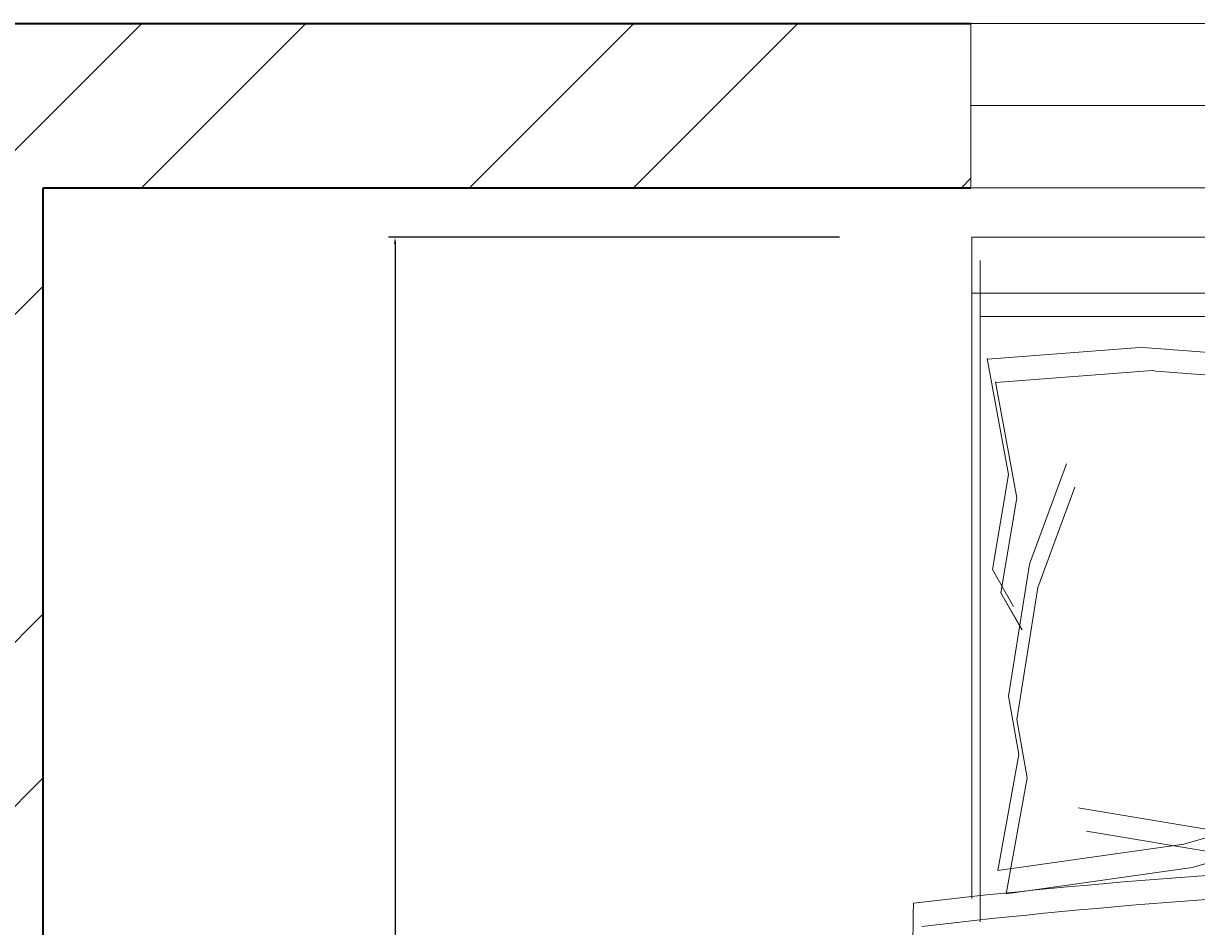
# Model space of a CAD drawing. Units: inches. Extents: x 1885 to 2748, y 783 to 2421.
# Tile 97 of 117: x 2363 to 2395, y 2328 to 2353. Entities that reach past the tile are written whole.
import ezdxf

# ---------------------------------------------------------------- set-up
doc = ezdxf.new("R2010")
doc.units = ezdxf.units.IN
for name, color, linetype, lineweight in [('A-ANNO-DIMS', 2, 'Continuous', 18), ('A-FURN', 8, 'Continuous', 13), ('A-GLAZ', 181, 'Continuous', 18), ('A-WALL', 7, 'Continuous', 35)]:
    doc.layers.add(name, color=color, linetype=linetype, lineweight=lineweight)
doc.layers.add('A-WALL-PATT', color=85, linetype='Continuous', lineweight=13, true_color=0x58ba48)
doc.styles.get("Standard").update_dxf_attribs({"font": 'arial.ttf'})
doc.dimstyles.get("Standard").update_dxf_attribs({"dimtxt": 0.18, "dimasz": 0.18, "dimexe": 0.18, "dimexo": 0.0625, "dimgap": 0.09, "dimtad": 0, "dimtih": 1, "dimtoh": 1, "dimdec": 4, "dimzin": 0, "dimdsep": 46, "dimtxsty": 'Standard', "dimcen": 0.09, "dimadec": 0, "dimazin": 0, "dimtfac": 1, "dimtdec": 4, "dimtofl": 0, "dimtmove": 0, "dimatfit": 3, "dimfxl": 1, "dimtolj": 1, "dimtzin": 0, "dimarcsym": 0})

# ---------------------------------------------------------------- blocks, each defined once
blk = doc.blocks.new('BED-DOUBLE')
for p, q in [((0.004, 3.474), (0.004, 51.493)), ((2.177, 3.702), (2.177, 51.493)), ((2.177, 3.702), (2.177, 51.492)), ((1.537, 3.474), (1.537, 51.264)), ((1.537, 3.474), (1.537, 51.264)), ((3.67, 8.512), (3.959, 12.335)), ((3.67, 8.512), (3.959, 12.335)), ((3.031, 8.284), (3.32, 12.107)), ((3.031, 8.283), (3.32, 12.107)), ((16.271, 6.609), (16.938, 10.641)), ((16.272, 6.609), (16.938, 10.64)), ((16.938, 10.641), (17.261, 9.508)), ((16.938, 10.64), (17.261, 9.507)), ((15.632, 6.38), (16.299, 10.412)), ((15.632, 6.38), (16.299, 10.412)), ((16.299, 10.412), (16.622, 9.279)), ((16.299, 10.412), (16.622, 9.279)), ((17.261, 9.508), (17.984, 4.411)), ((17.261, 9.507), (17.984, 4.411)), ((16.622, 9.279), (17.345, 4.183)), ((16.622, 9.279), (17.345, 4.182)), ((3.652, 8.407), (3.67, 8.512)), ((3.652, 8.406), (3.67, 8.512)), ((3.981, 4.126), (3.652, 8.407)), ((3.981, 4.125), (3.652, 8.406)), ((3.012, 8.178), (3.031, 8.284)), ((3.012, 8.178), (3.031, 8.283)), ((3.342, 3.897), (3.012, 8.178)), ((3.342, 3.897), (3.012, 8.178)), ((9.598, 5.278), (6.851, 6.29)), ((9.598, 5.278), (6.851, 6.29)), ((8.959, 5.05), (6.211, 6.062)), ((8.959, 5.05), (6.211, 6.061)), ((13.213, 4.7), (9.598, 5.278)), ((13.213, 4.7), (9.598, 5.278)), ((12.573, 4.472), (8.959, 5.05)), ((12.573, 4.471), (8.959, 5.05)), ((9.743, 4.266), (10.755, 4.845)), ((9.743, 4.266), (10.755, 4.844)), ((14.803, 4.989), (13.213, 4.7)), ((14.803, 4.989), (13.213, 4.7)), ((17.984, 4.411), (14.803, 4.989)), ((17.984, 4.411), (14.803, 4.989)), ((3.959, 4.122), (7.14, 4.7)), ((3.959, 4.121), (7.14, 4.7)), ((7.14, 4.7), (9.743, 4.266)), ((7.14, 4.7), (9.743, 4.266)), ((9.103, 4.038), (10.115, 4.616)), ((9.103, 4.038), (10.115, 4.616)), ((14.164, 4.761), (12.573, 4.472)), ((14.164, 4.76), (12.573, 4.471)), ((17.345, 4.183), (14.164, 4.761)), ((17.345, 4.182), (14.164, 4.76)), ((3.32, 3.893), (6.501, 4.472)), ((3.32, 3.893), (6.501, 4.471)), ((6.501, 4.472), (9.103, 4.038)), ((6.501, 4.471), (9.103, 4.038)), ((18.753, 3.702), (0.643, 3.702)), ((18.753, 3.702), (0.643, 3.702)), ((18.114, 3.474), (0.004, 3.474)), ((18.114, 3.474), (0.004, 3.474))]:
    blk.add_line(p, q)
for centre, radius, start, end in [((182.695, 21.586), 164.969, 176.08655, 186.78213), ((182.695, 21.586), 164.969, 176.08655, 186.78213), ((182.056, 21.358), 164.969, 176.08655, 186.78213), ((182.056, 21.357), 164.969, 176.08655, 186.78213), ((20.1, 85.16), 83.306, 268.72178, 275.60397), ((20.1, 85.16), 83.306, 268.72178, 275.60397)]:
    blk.add_arc(centre, radius, start, end)
blk = doc.blocks.new('WIN-60')
for p, q in [((0.004, 59.998), (0.004, -0.002)), ((2.254, 59.998), (2.254, -0.002)), ((4.504, -0.002), (4.504, 59.998)), ((2.254, -0.002), (0.004, -0.002)), ((0.004, -0.002), (4.504, -0.002))]:
    blk.add_line(p, q)
blk = doc.blocks.new('*D27')
at = {"layer": 'A-ANNO-DIMS', "color": 0, "lineweight": -2, "transparency": 16777216}
for p, q in [((2385.079, 2346.649), (2372.729, 2346.649)), ((2372.909, 2346.469), (2372.909, 2306.056)), ((2372.909, 2265.28), (2372.909, 2305.693)), ((2385.079, 2265.1), (2372.729, 2265.1))]:
    blk.add_line(p, q, dxfattribs=at)
at = {"layer": 'A-ANNO-DIMS', "color": 0, "transparency": 16777216}
for points in [[(2372.879, 2346.469), (2372.939, 2346.469), (2372.909, 2346.649)], [(2372.879, 2265.28), (2372.939, 2265.28), (2372.909, 2265.1)]]:
    blk.add_solid(points, dxfattribs=at)
at = {"layer": 'Defpoints', "color": 0, "transparency": 16777216}
for p in [(2385.141, 2346.649), (2372.909, 2265.1), (2385.141, 2265.1)]:
    blk.add_point(p, dxfattribs=at)
at = {"layer": 'A-ANNO-DIMS', "color": 0, "transparency": 16777216, "insert": (2372.909, 2305.874), "char_height": 0.18, "attachment_point": 5}
blk.add_mtext('\\A1;BED 82 TYP.', dxfattribs=at)

msp = doc.modelspace()

# ---------------------------------------------------------------- hatches: boundary and pattern name
at = {"layer": 'A-WALL-PATT'}
h = msp.add_hatch(dxfattribs=at)
h.set_pattern_fill('ANSI32', color=256)
h.paths.add_polyline_path([(2007.772, 2318.006), (1980.774, 2318.006), (1980.774, 2281.215), (1985.274, 2281.215), (1985.274, 2313.506), (2007.772, 2313.506), (2007.772, 2315.756)])
h.paths.add_polyline_path([(2094.324, 2318.006), (2067.772, 2318.006), (2067.772, 2313.506), (2094.324, 2313.506), (2094.324, 2315.756)])
h.paths.add_polyline_path([(2131.367, 2315.756), (2131.367, 2318.006), (2131.189, 2318.006), (2112.609, 2318.006), (2112.609, 2313.506), (2117.274, 2313.506), (2117.274, 2255.201), (2121.774, 2255.201), (2121.774, 2313.506), (2131.367, 2313.506)])
h.paths.add_polyline_path([(2190.512, 2318.006), (2155.367, 2318.006), (2155.367, 2313.506), (2169.774, 2313.506), (2169.774, 2229.506), (2121.774, 2229.506), (2121.774, 2233.451), (2119.524, 2233.451), (2117.274, 2233.451), (2117.274, 2201.101), (2121.774, 2201.101), (2121.774, 2225.006), (2169.774, 2225.006), (2169.774, 2165.006), (2306.274, 2165.006), (2306.274, 2066.006), (2310.774, 2066.006), (2344.274, 2066.006), (2486.274, 2066.006), (2486.274, 1886.006), (2483.02, 1886.006), (2483.02, 1881.506), (2486.274, 1881.506), (2486.274, 1880.678), (2490.774, 1880.678), (2490.774, 2070.506), (2344.274, 2070.506), (2310.774, 2070.506), (2310.774, 2165.006), (2310.774, 2173.636), (2308.524, 2173.636), (2306.274, 2173.636), (2306.274, 2169.506), (2174.274, 2169.506), (2174.274, 2313.506), (2190.512, 2313.506), (2190.512, 2315.756)])
h.paths.add_polyline_path([(1985.274, 2221.215), (1980.774, 2221.215), (1980.774, 2165.006), (1992.774, 2165.006), (1992.774, 2141.927), (1997.274, 2141.927), (1997.274, 2165.006), (2117.274, 2165.006), (2117.274, 2163.126), (2121.774, 2163.126), (2121.774, 2172.734), (2119.524, 2172.734), (2117.274, 2172.734), (2117.274, 2169.506), (1985.274, 2169.506)])
h.paths.add_polyline_path([(1997.274, 2105.927), (1992.774, 2105.927), (1992.774, 2070.506), (2016.774, 2070.506), (2016.774, 2059.123), (2019.024, 2059.123), (2021.274, 2059.123), (2021.274, 2070.506), (2117.274, 2070.506), (2117.274, 2022.506), (2114.423, 2022.506), (2114.423, 2018.006), (2123.627, 2018.006), (2123.627, 2020.256), (2123.627, 2022.506), (2121.774, 2022.506), (2121.774, 2142.587), (2119.524, 2142.587), (2117.274, 2142.587), (2117.274, 2075.006), (1997.274, 2075.006)])
h.paths.add_polyline_path([(2092.029, 2020.256), (2092.029, 2022.506), (2021.274, 2022.506), (2021.274, 2035.123), (2016.774, 2035.123), (2016.774, 2018.006), (2016.774, 1978.784), (2021.274, 1978.784), (2021.274, 2018.006), (2092.029, 2018.006)])
h.paths.add_polyline_path([(2260.938, 2022.506), (2153.105, 2022.506), (2153.105, 2020.256), (2153.105, 2018.006), (2155.274, 2018.006), (2155.274, 1886.006), (2107.629, 1886.006), (2107.629, 1881.506), (2182.911, 1881.506), (2182.911, 1883.756), (2182.911, 1886.006), (2159.774, 1886.006), (2159.774, 2018.006), (2260.938, 2018.006), (2260.938, 2020.256)])
h.paths.add_polyline_path([(2047.629, 1883.756), (2047.629, 1886.006), (2021.274, 1886.006), (2021.274, 1918.784), (2019.024, 1918.784), (2016.774, 1918.784), (2016.774, 1881.506), (2047.629, 1881.506)])
h.paths.add_polyline_path([(2306.361, 1883.756), (2306.361, 1886.006), (2296.274, 1886.006), (2296.274, 1982.006), (2316.535, 1982.006), (2316.535, 1984.256), (2316.535, 1986.506), (2296.274, 1986.506), (2296.274, 2022.506), (2289.276, 2022.506), (2289.276, 2018.006), (2291.774, 2018.006), (2291.774, 1886.006), (2242.911, 1886.006), (2242.911, 1881.506), (2306.361, 1881.506)], flags=17)
h.paths.add_polyline_path([(1985.274, 1843.006), (2021.6, 1843.006), (2021.534, 1845.441), (2021.477, 1847.506), (1980.774, 1847.506), (1980.774, 1809.446), (1985.274, 1809.446)])
h.paths.add_polyline_path([(2131.482, 1845.256), (2131.482, 1847.506), (2081.534, 1847.506), (2081.534, 1843.006), (2117.274, 1843.006), (2117.274, 1784.147), (2119.524, 1784.147), (2121.774, 1784.147), (2121.774, 1843.006), (2131.482, 1843.006)])
h.paths.add_polyline_path([(2203.886, 1847.506), (2155.482, 1847.506), (2155.482, 1843.006), (2169.774, 1843.006), (2169.774, 1759.006), (2121.774, 1759.006), (2121.774, 1761.457), (2117.274, 1761.457), (2117.274, 1730.429), (2121.774, 1730.429), (2121.774, 1754.506), (2177.421, 1754.506), (2177.421, 1756.756), (2177.421, 1759.006), (2174.274, 1759.006), (2174.274, 1843.006), (2203.886, 1843.006)])
h.paths.add_polyline_path([(2335.554, 1845.256), (2335.554, 1847.506), (2239.886, 1847.506), (2239.886, 1843.006), (2306.274, 1843.006), (2306.274, 1759.006), (2199.486, 1759.006), (2199.486, 1754.506), (2310.774, 1754.506), (2310.774, 1843.006), (2335.554, 1843.006)])
h.paths.add_polyline_path([(2348.774, 2022.506), (2344.274, 2022.506), (2344.274, 1986.506), (2341.681, 1986.506), (2341.681, 1982.006), (2344.274, 1982.006), (2344.274, 1886.006), (2330.361, 1886.006), (2330.361, 1881.506), (2361.627, 1881.506), (2361.627, 1883.756), (2361.627, 1886.006), (2348.774, 1886.006)], flags=17)
h.paths.add_polyline_path([(2283.251, 2315.756), (2283.251, 2318.006), (2238.512, 2318.006), (2238.512, 2313.506), (2283.251, 2313.506)], flags=17)
h.paths.add_polyline_path([(2363.274, 2348.006), (2388.677, 2348.006), (2388.677, 2350.256), (2388.677, 2352.506), (2358.774, 2352.506), (2358.774, 2348.006), (2358.774, 2318.006), (2344.481, 2318.006), (2344.481, 2313.506), (2358.774, 2313.506), (2358.774, 2229.506), (2310.774, 2229.506), (2310.774, 2231.952), (2306.274, 2231.952), (2306.274, 2205.611), (2310.774, 2205.611), (2310.774, 2225.006), (2358.774, 2225.006), (2358.774, 2211.506), (2452.329, 2211.506), (2452.329, 2213.756), (2452.329, 2216.006), (2363.274, 2216.006), (2363.274, 2318.006)])
h.paths.add_polyline_path([(2310.774, 2313.506), (2320.481, 2313.506), (2320.481, 2315.756), (2320.481, 2318.006), (2302.728, 2318.006), (2302.728, 2313.506), (2306.274, 2313.506), (2306.274, 2251.076), (2310.774, 2251.076)], flags=17)
h.paths.add_polyline_path([(2490.774, 2352.506), (2486.274, 2352.506), (2448.677, 2352.506), (2448.677, 2348.006), (2486.274, 2348.006), (2486.274, 2318.006), (2486.274, 2216.006), (2481.78, 2216.006), (2481.78, 2211.506), (2486.274, 2211.506), (2486.274, 2165.006), (2493.289, 2165.006), (2493.289, 2167.256), (2493.289, 2169.506), (2490.774, 2169.506), (2490.774, 2313.506), (2494.429, 2313.506), (2494.429, 2318.006), (2490.774, 2318.006)])
h.paths.add_polyline_path([(2534.653, 2318.006), (2515.691, 2318.006), (2515.691, 2313.506), (2534.653, 2313.506), (2534.653, 2315.756)])
h.paths.add_polyline_path([(2618.274, 2318.006), (2594.653, 2318.006), (2594.653, 2313.506), (2613.774, 2313.506), (2613.774, 2281.706), (2618.274, 2281.706)])
h.paths.add_polyline_path([(2618.274, 2221.706), (2613.774, 2221.706), (2613.774, 2169.506), (2554.019, 2169.506), (2554.019, 2165.006), (2613.774, 2165.006), (2613.774, 2152.878), (2618.274, 2152.878)])
h.paths.add_polyline_path([(2618.274, 2128.878), (2616.024, 2128.878), (2613.774, 2128.878), (2613.774, 2117.006), (2529.774, 2117.006), (2529.774, 2165.006), (2532.848, 2165.006), (2532.848, 2169.506), (2522.867, 2169.506), (2522.867, 2165.006), (2525.274, 2165.006), (2525.274, 2117.006), (2525.274, 2112.506), (2525.274, 2108.576), (2529.774, 2108.576), (2529.774, 2112.506), (2613.774, 2112.506), (2613.774, 2080.19), (2618.274, 2080.19)])
h.paths.add_polyline_path([(2618.274, 2044.19), (2616.024, 2044.19), (2613.774, 2044.19), (2613.774, 2015.506), (2529.774, 2015.506), (2529.774, 2088.582), (2527.524, 2088.582), (2525.274, 2088.582), (2525.274, 2011.006), (2613.774, 2011.006), (2613.774, 1956.755), (2618.274, 1956.755)])
h.paths.add_polyline_path([(2618.274, 1881.506), (2618.274, 1896.755), (2613.774, 1896.755), (2613.774, 1881.506), (2613.774, 1847.506), (2592.715, 1847.506), (2592.715, 1843.006), (2613.774, 1843.006), (2613.774, 1765.006), (2613.774, 1760.506), (2609.621, 1760.506), (2609.621, 1756.006), (2613.774, 1756.006), (2613.774, 1660.006), (2608.544, 1660.006), (2608.544, 1655.506), (2613.774, 1655.506), (2613.774, 1508.158), (2618.274, 1508.158)])
h.paths.add_polyline_path([(2565.774, 1843.006), (2568.997, 1843.006), (2568.997, 1847.506), (2490.774, 1847.506), (2490.774, 1849.7), (2488.524, 1849.7), (2486.274, 1849.7), (2486.274, 1847.506), (2477.274, 1847.506), (2477.274, 1838.506), (2477.274, 1821.493), (2486.274, 1821.493), (2486.274, 1838.506), (2561.274, 1838.506), (2561.274, 1765.006), (2486.274, 1765.006), (2486.274, 1786.157), (2477.274, 1786.157), (2477.274, 1765.006), (2477.274, 1756.006), (2486.274, 1756.006), (2565.774, 1756.006), (2585.621, 1756.006), (2585.621, 1758.256), (2585.621, 1760.506), (2565.774, 1760.506), (2565.774, 1765.006)])
h.paths.add_polyline_path([(2486.274, 1651.006), (2561.274, 1651.006), (2561.274, 1567.006), (2486.274, 1567.006), (2486.274, 1591.321), (2477.274, 1591.321), (2477.274, 1567.006), (2477.274, 1558.006), (2477.274, 1555.439), (2481.774, 1555.439), (2481.774, 1558.006), (2568.653, 1558.006), (2568.653, 1560.256), (2568.653, 1562.506), (2565.774, 1562.506), (2565.774, 1655.506), (2584.544, 1655.506), (2584.544, 1657.756), (2584.544, 1660.006), (2565.774, 1660.006), (2486.274, 1660.006), (2477.274, 1660.006), (2477.274, 1651.006), (2477.274, 1632.989), (2486.274, 1632.989)])
h.paths.add_polyline_path([(2449.967, 1883.756), (2449.967, 1886.006), (2421.627, 1886.006), (2421.627, 1881.506), (2449.967, 1881.506)], flags=17)
h.paths.add_polyline_path([(2447.274, 1847.506), (2395.554, 1847.506), (2395.554, 1843.006), (2442.774, 1843.006), (2442.774, 1809.27), (2447.274, 1809.27)])
h.paths.add_polyline_path([(1985.274, 1749.446), (1980.774, 1749.446), (1980.774, 1694.504), (1985.274, 1694.504), (1985.274, 1694.506), (1986.897, 1694.506), (1986.897, 1697.78), (1986.897, 1699.006), (1985.274, 1699.006)])
h.paths.add_polyline_path([(2152.774, 1699.006), (2121.774, 1699.006), (2121.774, 1703.668), (2119.524, 1703.668), (2117.274, 1703.668), (2117.274, 1699.006), (2009.219, 1699.006), (2009.219, 1694.506), (2148.274, 1694.506), (2148.274, 1692.631), (2152.774, 1692.631)])
h.paths.add_polyline_path([(2016.274, 1694.506), (2011.774, 1694.506), (2011.774, 1558.006), (2040.806, 1558.006), (2040.806, 1560.256), (2040.806, 1562.506), (2016.274, 1562.506)])
h.paths.add_polyline_path([(2152.774, 1663.017), (2150.524, 1663.017), (2148.274, 1663.017), (2148.274, 1562.506), (2100.806, 1562.506), (2100.806, 1558.006), (2165.119, 1558.006), (2165.119, 1560.256), (2165.119, 1562.506), (2152.774, 1562.506), (2152.774, 1610.506), (2224.774, 1610.506), (2224.774, 1607.99), (2229.274, 1607.99), (2229.274, 1615.006), (2152.774, 1615.006)])
h.paths.add_polyline_path([(2238.613, 1560.256), (2238.613, 1562.506), (2229.274, 1562.506), (2229.274, 1588.756), (2227.024, 1588.763), (2224.774, 1588.771), (2224.774, 1562.506), (2189.119, 1562.506), (2189.119, 1558.006), (2238.613, 1558.006)])
h.paths.add_polyline_path([(2336.024, 1560.256), (2336.024, 1562.506), (2310.774, 1562.506), (2310.774, 1656.347), (2308.524, 1656.347), (2306.274, 1656.347), (2306.274, 1562.506), (2286.613, 1562.506), (2286.613, 1558.006), (2336.024, 1558.006)])
h.paths.add_polyline_path([(2447.274, 1690.968), (2445.024, 1690.968), (2442.774, 1690.968), (2442.774, 1687.006), (2306.274, 1687.006), (2306.274, 1680.75), (2310.774, 1680.75), (2310.774, 1682.506), (2442.774, 1682.506), (2442.774, 1562.506), (2396.024, 1562.506), (2396.024, 1558.006), (2447.274, 1558.006)])
h.paths.add_polyline_path([(2447.274, 1749.27), (2445.024, 1749.27), (2442.774, 1749.27), (2442.774, 1717.232), (2447.274, 1717.232)])
h.paths.add_polyline_path([(2044.674, 1521.756), (2044.674, 1524.006), (2007.274, 1524.006), (2007.274, 1503.49), (2009.524, 1503.49), (2011.774, 1503.49), (2011.774, 1519.506), (2044.674, 1519.506)])
h.paths.add_polyline_path([(2177.969, 1521.756), (2177.969, 1524.006), (2104.674, 1524.006), (2104.674, 1519.506), (2145.774, 1519.506), (2145.774, 1387.506), (2143.37, 1387.506), (2143.37, 1383.006), (2251.585, 1383.006), (2251.585, 1385.256), (2251.585, 1387.506), (2150.274, 1387.506), (2150.274, 1519.506), (2177.969, 1519.506)])
h.paths.add_polyline_path([(2298.704, 1524.006), (2237.969, 1524.006), (2237.969, 1519.506), (2282.274, 1519.506), (2282.274, 1387.506), (2279.683, 1387.506), (2279.683, 1383.006), (2286.774, 1383.006), (2286.774, 1419.006), (2312.451, 1419.006), (2312.451, 1421.256), (2312.451, 1423.506), (2286.774, 1423.506), (2286.774, 1519.506), (2298.704, 1519.506), (2298.704, 1521.722)], flags=17)
h.paths.add_polyline_path([(2361.897, 1521.756), (2361.897, 1524.006), (2322.704, 1524.006), (2322.704, 1519.506), (2334.774, 1519.506), (2334.774, 1423.506), (2331.93, 1423.506), (2331.93, 1419.006), (2334.774, 1419.006), (2334.774, 1387.506), (2334.774, 1383.228), (2339.274, 1383.228), (2339.274, 1387.506), (2339.274, 1519.506), (2361.897, 1519.506)], flags=17)
h.paths.add_polyline_path([(2447.274, 1521.756), (2447.274, 1524.006), (2421.897, 1524.006), (2421.897, 1519.506), (2447.274, 1519.506)], flags=17)
h.paths.add_polyline_path([(2481.774, 1529.6), (2479.524, 1529.6), (2477.274, 1529.6), (2477.274, 1524.006), (2474.489, 1524.006), (2474.489, 1519.506), (2477.274, 1519.506), (2477.274, 1334.506), (2296.774, 1334.506), (2296.774, 1240.506), (2160.274, 1240.506), (2160.274, 1180.506), (2112.274, 1180.506), (2112.274, 1207.692), (2110.024, 1207.692), (2107.774, 1207.692), (2107.774, 1171.609), (2112.274, 1171.609), (2112.274, 1176.006), (2160.274, 1176.006), (2160.274, 1092.006), (2144.221, 1092.006), (2144.221, 1087.506), (2189.497, 1087.506), (2189.497, 1089.756), (2189.497, 1092.006), (2164.774, 1092.006), (2164.774, 1236.006), (2296.774, 1236.006), (2296.774, 1231.912), (2301.274, 1231.912), (2301.274, 1330.006), (2481.774, 1330.006), (2481.774, 1387.506)])
h.paths.add_polyline_path([(2618.274, 1448.158), (2613.774, 1448.158), (2613.774, 1382.506), (2529.774, 1382.506), (2525.274, 1382.506), (2525.274, 1307.062), (2529.774, 1307.062), (2529.774, 1378.006), (2613.774, 1378.006), (2613.774, 1354.988), (2618.274, 1354.988)])
h.paths.add_polyline_path([(2618.274, 1318.988), (2613.774, 1318.988), (2613.774, 1281.006), (2529.774, 1281.006), (2529.774, 1283.786), (2527.524, 1283.786), (2525.274, 1283.786), (2525.274, 1228.506), (2516.794, 1228.506), (2516.794, 1224.006), (2533.484, 1224.006), (2533.484, 1226.256), (2533.484, 1228.506), (2529.774, 1228.506), (2529.774, 1276.506), (2613.774, 1276.506), (2613.774, 1266.02), (2618.274, 1266.02)])
h.paths.add_polyline_path([(2618.274, 1134.964), (2613.774, 1134.964), (2613.774, 1092.006), (2594.545, 1092.006), (2594.545, 1087.506), (2618.274, 1087.506)])
h.paths.add_polyline_path([(2534.545, 1092.006), (2509.765, 1092.006), (2509.765, 1087.506), (2534.545, 1087.506), (2534.545, 1089.756)])
h.paths.add_polyline_path([(2481.274, 1224.006), (2484.117, 1224.006), (2484.117, 1226.256), (2484.117, 1228.506), (2476.774, 1228.506), (2476.774, 1198.506), (2471.61, 1198.506), (2471.61, 1194.006), (2476.774, 1194.006), (2476.774, 1062.006), (2436.894, 1062.006), (2436.894, 1057.506), (2476.774, 1057.506), (2481.274, 1057.506), (2481.274, 1062.006), (2481.274, 1087.506), (2485.354, 1087.506), (2485.354, 1089.756), (2485.354, 1092.006), (2481.274, 1092.006), (2481.274, 1117.506)])
h.paths.add_polyline_path([(2439.898, 1198.506), (2349.274, 1198.506), (2349.274, 1194.006), (2349.274, 1180.506), (2301.274, 1180.506), (2301.274, 1201.896), (2299.024, 1201.896), (2296.774, 1201.896), (2296.774, 1172.335), (2299.024, 1172.335), (2301.274, 1172.335), (2301.274, 1176.006), (2349.274, 1176.006), (2349.274, 1092.006), (2334.452, 1092.006), (2334.452, 1087.506), (2349.274, 1087.506), (2349.274, 1057.506), (2353.774, 1057.506), (2376.894, 1057.506), (2376.894, 1059.756), (2376.894, 1062.006), (2353.774, 1062.006), (2353.774, 1087.506), (2353.774, 1180.506), (2353.774, 1194.006), (2439.898, 1194.006), (2439.898, 1196.256)])
h.paths.add_polyline_path([(2270.596, 1089.756), (2270.596, 1092.006), (2249.497, 1092.006), (2249.497, 1087.506), (2270.596, 1087.506)], flags=17)
h.paths.add_polyline_path([(2310.452, 1092.006), (2301.274, 1092.006), (2301.274, 1153.292), (2296.774, 1153.292), (2296.774, 1092.006), (2293.786, 1092.006), (2293.786, 1087.506), (2310.452, 1087.506), (2310.452, 1089.756)], flags=17)
h.paths.add_polyline_path([(2112.274, 1150.328), (2110.024, 1150.328), (2107.774, 1150.328), (2107.774, 1092.006), (2104.465, 1092.006), (2104.465, 1087.506), (2120.221, 1087.506), (2120.221, 1089.756), (2120.221, 1092.006), (2112.274, 1092.006)])
h.paths.add_polyline_path([(2082.172, 1092.006), (2058.144, 1092.006), (2058.144, 1087.506), (2082.172, 1087.506), (2082.172, 1089.756)])
h.paths.add_polyline_path([(1975.774, 1145.638), (1971.274, 1145.638), (1971.274, 1087.506), (1980.774, 1087.506), (1998.144, 1087.506), (1998.144, 1089.756), (1998.144, 1092.006), (1985.274, 1092.006), (1975.774, 1092.006)])
h.paths.add_polyline_path([(2112.274, 1244.385), (2110.024, 1244.385), (2107.774, 1244.385), (2107.774, 1240.506), (1992.274, 1240.506), (1992.274, 1271.008), (1987.774, 1271.008), (1987.774, 1240.506), (1980.774, 1240.506), (1975.774, 1240.506), (1971.274, 1240.506), (1971.274, 1205.638), (1975.774, 1205.638), (1975.774, 1236.006), (2107.774, 1236.006), (2107.774, 1233.444), (2112.274, 1233.444), (2112.274, 1236.006)])
h.paths.add_polyline_path([(2112.274, 1383.006), (2114.783, 1383.006), (2114.783, 1385.256), (2114.783, 1387.506), (2102.476, 1387.506), (2102.476, 1383.006), (2107.774, 1383.006), (2107.774, 1335.006), (2011.774, 1335.006), (2011.774, 1349.939), (2007.274, 1349.939), (2007.274, 1335.006), (1987.774, 1335.006), (1987.774, 1330.506), (1987.774, 1307.008), (1992.274, 1307.008), (1992.274, 1330.506), (2007.274, 1330.506), (2107.774, 1330.506), (2107.774, 1264.711), (2112.274, 1264.711)])
h.paths.add_polyline_path([(2077.857, 1387.506), (2011.774, 1387.506), (2011.774, 1390.036), (2009.524, 1390.036), (2007.274, 1390.036), (2007.274, 1373.939), (2011.774, 1373.939), (2011.774, 1383.006), (2077.857, 1383.006)])
h.paths.add_polyline_path([(2011.774, 1443.49), (2007.274, 1443.49), (2007.274, 1410.248), (2011.774, 1410.248)])

# ---------------------------------------------------------------- linework, layer by layer
at = {"layer": 'A-WALL'}
for p, q in [((2358.774, 2352.506), (2388.677, 2352.506)), ((2363.274, 2318.006), (2363.274, 2348.006)), ((2363.274, 2348.006), (2388.677, 2348.006))]:
    msp.add_line(p, q, dxfattribs=at)

# ---------------------------------------------------------------- block references
at = {"layer": 'A-FURN', "rotation": 269.9999998331857}
msp.add_blockref('BED-DOUBLE', (2385.229, 2346.652), dxfattribs=at)
at = {"layer": 'A-GLAZ', "extrusion": (0, 0, -1), "zscale": -1, "rotation": 90}
msp.add_blockref('WIN-60', (-2388.679, 2348.002), dxfattribs=at)

# ---------------------------------------------------------------- dimensions: what is measured, and where the dimension line sits
at = {"layer": 'A-ANNO-DIMS'}
dim = msp.add_linear_dim(base=(2372.909, 2265.1), p1=(2385.141, 2346.649), p2=(2385.141, 2265.1), angle=270, text='BED <> TYP.', dimstyle='Standard', override={"dimdec": 0, "dimlfac": 1, "dimrnd": 0, "dimzin": 0, "dimdsep": 46, "dimlunit": 2}, dxfattribs=at)
dim.commit()
dim.dimension.update_dxf_attribs({"geometry": '*D27', "text_midpoint": (2372.909, 2305.874)})

doc.saveas('drawing.dxf')
